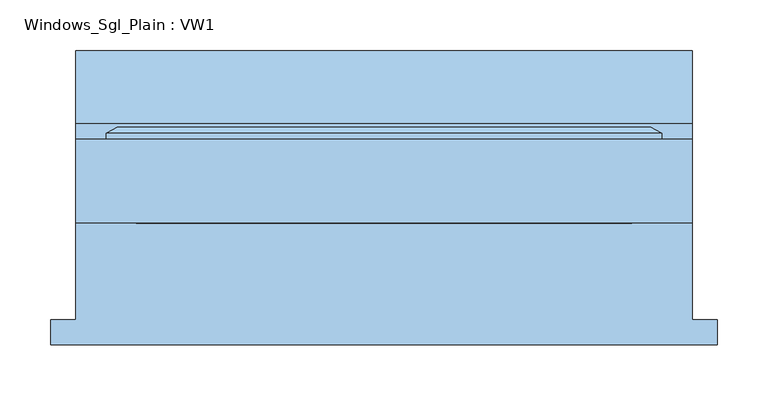
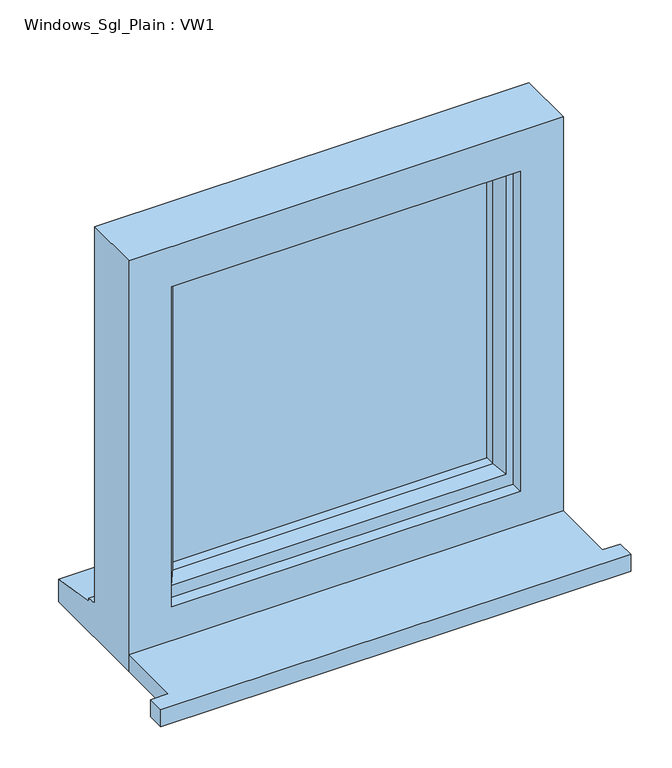
"""IFC4 building model written with IfcOpenShell, lengths in millimetres: window geometry, Windows_Sgl_Plain : VW1."""

from ifc_helpers import new_model, si_unit, frame, origin, place, context, project, spatial, polyline, outline, extrude, faceted_brep, source, transform, mapped, element, save


def windows_sgl_plain_vw1_399019d4(model_context):
    return source(origin(), model_context, "Body", "SolidModel", [
        extrude(outline(polyline([(-329.8, -130.8434322), (-329.8, -105.8434322), (-304.8, -105.8434322), (-304.8, -10.2434322), (304.8, -10.2434322), (304.8, -105.8434322), (329.8, -105.8434322), (329.8, -130.8434322), (-329.8, -130.8434322)])), frame((0.0, 0.0, 1500.4), z_axis=(0.0, 0.0, 1.0), x_axis=(1.0, 0.0, 0.0)), (0.0, 0.0, 1.0), 25.0),
        faceted_brep([(-274.8, 72.7565678, 2080.0), (-274.8, 78.5300705, 2080.0), (-274.8, 78.5300705, 1553.4), (-274.8, 72.7565678, 1553.4), (-264.8, 7.7565678, 2070.0), (-264.8, 72.7565678, 2070.0), (-264.8, 72.7565678, 1563.4), (-264.8, 7.7565678, 1563.4), (-224.8, 22.2494677, 2030.0), (-234.9480377, 7.7565678, 2040.1480377), (-234.9480377, 7.7565678, 1593.2519623), (-224.8, 22.2494677, 1603.4), (-224.8, 36.7565678, 2030.0), (-224.8, 36.7565678, 1603.4), (-234.8, 60.7565678, 2040.0), (-234.8, 36.7565678, 2040.0), (-234.8, 36.7565678, 1593.4), (-234.8, 60.7565678, 1593.4), (-224.8, 78.5300705, 2030.0), (-224.8, 60.7565678, 2030.0), (-224.8, 60.7565678, 1603.4), (-224.8, 78.5300705, 1603.4), (-242.2457548, 84.3035732, 2047.4457548), (-242.2457548, 84.3035732, 1585.9542452), (-264.0153903, 84.3035732, 2069.2153903), (-264.0153903, 84.3035732, 1564.1846097), (274.8, 78.5300705, 1553.4), (274.8, 72.7565678, 1553.4), (264.8, 72.7565678, 1563.4), (264.8, 7.7565678, 1563.4), (234.9480377, 7.7565678, 1593.2519623), (224.8, 22.2494677, 1603.4), (224.8, 36.7565678, 1603.4), (234.8, 36.7565678, 1593.4), (234.8, 60.7565678, 1593.4), (224.8, 60.7565678, 1603.4), (224.8, 78.5300705, 1603.4), (242.2457548, 84.3035732, 1585.9542452), (264.0153903, 84.3035732, 1564.1846097), (274.8, 78.5300705, 2080.0), (274.8, 72.7565678, 2080.0), (264.8, 72.7565678, 2070.0), (264.8, 7.7565678, 2070.0), (234.9480377, 7.7565678, 2040.1480377), (224.8, 22.2494677, 2030.0), (224.8, 36.7565678, 2030.0), (234.8, 36.7565678, 2040.0), (234.8, 60.7565678, 2040.0), (224.8, 60.7565678, 2030.0), (224.8, 78.5300705, 2030.0), (242.2457548, 84.3035732, 2047.4457548), (264.0153903, 84.3035732, 2069.2153903)], [[[0, 1, 2, 3]], [[4, 5, 6, 7]], [[8, 9, 10, 11]], [[12, 8, 11, 13]], [[14, 15, 16, 17]], [[18, 19, 20, 21]], [[22, 18, 21, 23]], [[1, 24, 25, 2]], [[3, 2, 26, 27]], [[7, 6, 28, 29]], [[11, 10, 30, 31]], [[13, 11, 31, 32]], [[17, 16, 33, 34]], [[21, 20, 35, 36]], [[23, 21, 36, 37]], [[2, 25, 38, 26]], [[27, 26, 39, 40]], [[29, 28, 41, 42]], [[31, 30, 43, 44]], [[32, 31, 44, 45]], [[34, 33, 46, 47]], [[36, 35, 48, 49]], [[37, 36, 49, 50]], [[26, 38, 51, 39]], [[40, 39, 1, 0]], [[3, 27, 40, 0], [5, 41, 28, 6]], [[42, 41, 5, 4]], [[7, 29, 42, 4], [9, 43, 30, 10]], [[44, 43, 9, 8]], [[45, 44, 8, 12]], [[15, 46, 33, 16], [13, 32, 45, 12]], [[47, 46, 15, 14]], [[17, 34, 47, 14], [19, 48, 35, 20]], [[49, 48, 19, 18]], [[50, 49, 18, 22]], [[24, 51, 38, 25], [23, 37, 50, 22]], [[39, 51, 24, 1]]]),
        extrude(outline(polyline([(234.8, 36.7565678), (-234.8, 36.7565678), (-234.8, 60.7565678), (234.8, 60.7565678), (234.8, 36.7565678)])), frame((0.0, 0.0, 1593.4), z_axis=(0.0, 0.0, 1.0), x_axis=(1.0, 0.0, 0.0)), (0.0, 0.0, 1.0), 446.6),
        faceted_brep([(-304.8, -10.2434322, 1500.4), (304.8, -10.2434322, 1500.4), (304.8, -10.2434322, 2110.0), (-304.8, -10.2434322, 2110.0), (-244.8, -10.2434322, 2050.0), (244.8, -10.2434322, 2050.0), (244.8, -10.2434322, 1575.4), (-244.8, -10.2434322, 1575.4), (-304.8, 72.7565678, 2110.0), (-304.8, 72.7565678, 1551.4), (-304.8, 87.7565678, 1550.08767), (-304.8, 87.7565678, 1545.1449676), (-304.8, 160.2565678, 1534.2088847), (-304.8, 160.2565678, 1500.4), (304.8, 72.7565678, 2110.0), (304.8, 72.7565678, 1551.4), (-264.8, 72.7565678, 2070.0), (-264.8, 72.7565678, 1563.4), (264.8, 72.7565678, 1563.4), (264.8, 72.7565678, 2070.0), (-264.8, 7.7565678, 2070.0), (-264.8, 7.7565678, 1563.4), (264.8, 7.7565678, 2070.0), (264.8, 7.7565678, 1563.4), (-244.8, 7.7565678, 2050.0), (-244.8, 7.7565678, 1575.4), (244.8, 7.7565678, 1575.4), (244.8, 7.7565678, 2050.0), (304.8, 160.2565678, 1500.4), (304.8, 160.2565678, 1534.2088847), (304.8, 87.7565678, 1545.1449676), (304.8, 87.7565678, 1550.08767)], [[[0, 1, 2, 3], [4, 5, 6, 7]], [[0, 3, 8, 9, 10, 11, 12, 13]], [[9, 8, 14, 15], [16, 17, 18, 19]], [[17, 16, 20, 21]], [[20, 22, 23, 21], [24, 25, 26, 27]], [[24, 4, 7, 25]], [[3, 2, 14, 8]], [[16, 19, 22, 20]], [[5, 4, 24, 27]], [[15, 14, 2, 1, 28, 29, 30, 31]], [[19, 18, 23, 22]], [[5, 27, 26, 6]], [[28, 1, 0, 13]], [[29, 28, 13, 12]], [[30, 29, 12, 11]], [[31, 30, 11, 10]], [[15, 31, 10, 9]], [[21, 23, 18, 17]], [[7, 6, 26, 25]]]),
    ])


if __name__ == "__main__":
    model = new_model("IFC4")
    model_context = context("Model", 3, world=origin())
    ifc_project = project(units=[si_unit("LENGTHUNIT", "METRE", prefix="MILLI")], contexts=[model_context])
    site = spatial("IfcSite", under=ifc_project)
    building = spatial("IfcBuilding", under=site)
    placement = place(None, origin())
    windows_sgl_plain_vw1_shape = windows_sgl_plain_vw1_399019d4(model_context)
    element("IfcWindow", 1, ObjectType="Windows_Sgl_Plain : VW1", at=placement, inside=building, context=model_context, shape_type="MappedRepresentation", body=[
        mapped(windows_sgl_plain_vw1_shape, transform((0.0, 0.0, 0.0), x_axis=(1.0, 0.0, 0.0), y_axis=(0.0, 1.0, 0.0), z_axis=(0.0, 0.0, 1.0))),
    ])
    save(model, "model.ifc")

# Revit data of these elements
# Type "Windows_Sgl_Plain : VW1"
#   Type Mark = "64"
#   Operation = "SinglePanel"
#   Construction Type Id = "SGL"
#   Manufacturer = "Revit"
#   Keynote = "L10"
#   Analytic Construction = "Large single-glazed windows"
#   Wrap Layers (Ext) from Ext = 0.336286 ft
#   Wrap Layers (Int) from Ext = 0.582349 ft
#   Window Board Projection = 0.082021 ft
#   Window Board Extension = 0.082021 ft
#   Visual Light Transmittance = 0.9
#   Solar Heat Gain Coefficient = 0.86
#   Rough Width = 2.0 ft
#   Rough Height = 2.0 ft
#   Height = 2.0 ft
#   Width = 2.0 ft
#   Heat Transfer Coefficient (U) = 5.5617 W/(m²·K)
#   Glazing Thickness = 0.07874 ft
#   FrameOffset - External = 0.164042 ft
#   Frame Depth = 0.213255 ft
#   Default Head Height = 6.922572 ft
#   Cill Depth = 0.287073 ft
#   Cavity Closer Width = 0.164042 ft
#   Cavity Closer Offset from Ext = 0.336286 ft
#   Cavity Closer Depth = 0.278871 ft
#   Vis - Cavity Closers = yes
#   Define Thermal Properties by = 1
#   Material Trim = Window Frame
#   Material Glass = Glass
#   Material Frame = Window Frame
#   Wall Closure = (empty or 0)
# Element 1 (IfcWindow, "Windows_Sgl_Plain : VW1")
#   Materials on its faces: "Window Frame", "Glass"
# Materials
#   "Window Frame": colour RGB 249 249 249, transparency 0, Keynote = "L10", Cost = 0
#   "Glass": class "Glass", colour RGB 0 128 192, transparency 0.9, Description = "Soda Lime Glass", Cost = 0
